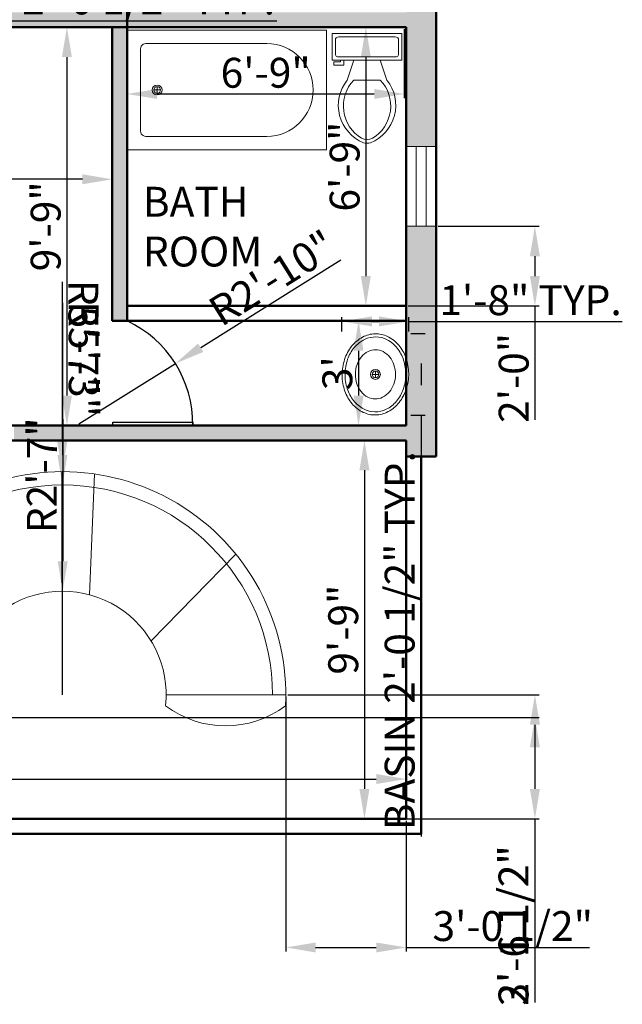
# Model space of a CAD drawing. Units: inches. Extents: x 875413 to 876020, y 447446 to 448210.
# Tile 4 of 8: x 875810 to 875992, y 447498 to 447795. Entities that reach past the tile are written whole.
import ezdxf

# ---------------------------------------------------------------- set-up
doc = ezdxf.new("R2010")
doc.units = ezdxf.units.IN
for name, color, linetype, lineweight in [('A-ANNO-DIMS', 2, 'Continuous', 13), ('A-AREA-IDEN', 7, 'Continuous', 25), ('A-DOOR', 3, 'Continuous', 25), ('A-FLOR-FIXT', 9, 'Continuous', 18), ('A-FURN', 8, 'Continuous', 18), ('A-GLAZ', 4, 'Continuous', 20), ('A-WALL', 7, 'Continuous', 50)]:
    doc.layers.add(name, color=color, linetype=linetype, lineweight=lineweight)
doc.layers.add('A-WALL-PATT', color=18, linetype='Continuous', lineweight=13, true_color=0x000000)
doc.styles.get("Standard").update_dxf_attribs({"font": 'arial.ttf'})
doc.dimstyles.new('ISO-25', dxfattribs={"dimtxt": 9, "dimasz": 9, "dimexe": 1.25, "dimexo": 0.625, "dimtad": 1, "dimdec": 1, "dimrnd": 9, "dimlunit": 3, "dimtxsty": 'Standard', "dimcen": 2.5, "dimadec": 0, "dimazin": 0, "dimtfac": 1, "dimtdec": 1, "dimtmove": 0, "dimatfit": 3, "dimfxl": 1, "dimarcsym": 0})

# ---------------------------------------------------------------- blocks, each defined once
blk = doc.blocks.new('*D19')
at = {"layer": 'A-ANNO-DIMS', "color": 0, "lineweight": -2, "transparency": 16777216}
for p, q in [((875643.2, 447554.64), (875643.2, 447567.26)), ((875652.2, 447566.01), (875917.7, 447566.01)), ((875926.7, 447554.64), (875926.7, 447567.26))]:
    blk.add_line(p, q, dxfattribs=at)
at = {"layer": 'A-ANNO-DIMS', "color": 0, "transparency": 16777216}
for points in [[(875652.2, 447567.51), (875652.2, 447564.51), (875643.2, 447566.01)], [(875917.7, 447567.51), (875917.7, 447564.51), (875926.7, 447566.01)]]:
    blk.add_solid(points, dxfattribs=at)
at = {"layer": 'Defpoints', "color": 0, "transparency": 16777216}
for p in [(875926.7, 447566.01), (875643.2, 447554.02), (875926.7, 447554.02)]:
    blk.add_point(p, dxfattribs=at)
at = {"layer": 'A-ANNO-DIMS', "color": 0, "transparency": 16777216, "insert": (875784.95, 447571.15), "char_height": 9, "attachment_point": 5}
blk.add_mtext("24'", dxfattribs=at)
blk = doc.blocks.new('*D20')
at = {"layer": 'A-ANNO-DIMS', "color": 0, "lineweight": -2, "transparency": 16777216}
for p, q in [((875926.08, 447668.02), (875912.88, 447668.02)), ((875914.13, 447659.02), (875914.13, 447563.02)), ((875926.08, 447554.02), (875912.88, 447554.02))]:
    blk.add_line(p, q, dxfattribs=at)
at = {"layer": 'A-ANNO-DIMS', "color": 0, "transparency": 16777216}
for points in [[(875912.63, 447659.02), (875915.63, 447659.02), (875914.13, 447668.02)], [(875912.63, 447563.02), (875915.63, 447563.02), (875914.13, 447554.02)]]:
    blk.add_solid(points, dxfattribs=at)
at = {"layer": 'Defpoints', "color": 0, "transparency": 16777216}
for p in [(875926.7, 447668.02), (875914.13, 447554.02), (875926.7, 447554.02)]:
    blk.add_point(p, dxfattribs=at)
at = {"layer": 'A-ANNO-DIMS', "color": 0, "transparency": 16777216, "insert": (875908.91, 447611.02), "char_height": 9, "attachment_point": 5, "rotation": 90}
blk.add_mtext('9\'-9"', dxfattribs=at)
blk = doc.blocks.new('*D21')
at = {"layer": 'A-ANNO-DIMS', "color": 0, "lineweight": -2, "transparency": 16777216}
for p, q in [((875926.08, 447792.52), (875913.3, 447792.52)), ((875914.55, 447783.52), (875914.55, 447717.52)), ((875926.08, 447708.52), (875913.3, 447708.52))]:
    blk.add_line(p, q, dxfattribs=at)
at = {"layer": 'A-ANNO-DIMS', "color": 0, "transparency": 16777216}
for points in [[(875913.05, 447783.52), (875916.05, 447783.52), (875914.55, 447792.52)], [(875913.05, 447717.52), (875916.05, 447717.52), (875914.55, 447708.52)]]:
    blk.add_solid(points, dxfattribs=at)
at = {"layer": 'Defpoints', "color": 0, "transparency": 16777216}
for p in [(875926.7, 447792.52), (875914.55, 447708.52), (875926.7, 447708.52)]:
    blk.add_point(p, dxfattribs=at)
at = {"layer": 'A-ANNO-DIMS', "color": 0, "transparency": 16777216, "insert": (875909.33, 447750.52), "char_height": 9, "attachment_point": 5, "rotation": 90}
blk.add_mtext('6\'-9"', dxfattribs=at)
blk = doc.blocks.new('*D22')
at = {"layer": 'A-ANNO-DIMS', "color": 0, "lineweight": -2, "transparency": 16777216}
for p, q in [((875842.7, 447791.89), (875842.7, 447771.14)), ((875926.08, 447791.89), (875926.08, 447771.14)), ((875851.7, 447772.39), (875917.08, 447772.39))]:
    blk.add_line(p, q, dxfattribs=at)
at = {"layer": 'A-ANNO-DIMS', "color": 0, "transparency": 16777216}
for points in [[(875851.7, 447773.89), (875851.7, 447770.89), (875842.7, 447772.39)], [(875917.08, 447773.89), (875917.08, 447770.89), (875926.08, 447772.39)]]:
    blk.add_solid(points, dxfattribs=at)
at = {"layer": 'Defpoints', "color": 0, "transparency": 16777216}
for p in [(875842.7, 447792.52), (875926.08, 447792.52), (875926.08, 447772.39)]:
    blk.add_point(p, dxfattribs=at)
at = {"layer": 'A-ANNO-DIMS', "color": 0, "transparency": 16777216, "insert": (875884.39, 447777.61), "char_height": 9, "attachment_point": 5}
blk.add_mtext('6\'-9"', dxfattribs=at)
blk = doc.blocks.new('*D23')
at = {"layer": 'A-ANNO-DIMS', "color": 0, "lineweight": -2, "transparency": 16777216}
for p, q in [((875926.08, 447704.02), (875911.11, 447704.02)), ((875912.36, 447695.02), (875912.36, 447681.52)), ((875926.08, 447672.52), (875911.11, 447672.52))]:
    blk.add_line(p, q, dxfattribs=at)
at = {"layer": 'A-ANNO-DIMS', "color": 0, "transparency": 16777216}
for points in [[(875910.86, 447695.02), (875913.86, 447695.02), (875912.36, 447704.02)], [(875910.86, 447681.52), (875913.86, 447681.52), (875912.36, 447672.52)]]:
    blk.add_solid(points, dxfattribs=at)
at = {"layer": 'Defpoints', "color": 0, "transparency": 16777216}
for p in [(875926.7, 447704.02), (875912.36, 447672.52), (875926.7, 447672.52)]:
    blk.add_point(p, dxfattribs=at)
at = {"layer": 'A-ANNO-DIMS', "color": 0, "transparency": 16777216, "insert": (875907.14, 447688.27), "char_height": 9, "attachment_point": 5, "rotation": 90}
blk.add_mtext("3'", dxfattribs=at)
blk = doc.blocks.new('*D24')
at = {"layer": 'A-ANNO-DIMS', "color": 0, "lineweight": -2, "transparency": 16777216}
for p, q in [((875689.7, 447791.89), (875689.7, 447745.44)), ((875838.2, 447791.89), (875838.2, 447745.44)), ((875829.2, 447746.69), (875698.7, 447746.69))]:
    blk.add_line(p, q, dxfattribs=at)
at = {"layer": 'A-ANNO-DIMS', "color": 0, "transparency": 16777216}
for points in [[(875698.7, 447748.19), (875698.7, 447745.19), (875689.7, 447746.69)], [(875829.2, 447748.19), (875829.2, 447745.19), (875838.2, 447746.69)]]:
    blk.add_solid(points, dxfattribs=at)
at = {"layer": 'Defpoints', "color": 0, "transparency": 16777216}
for p in [(875689.7, 447792.52), (875838.2, 447792.52), (875689.7, 447746.69)]:
    blk.add_point(p, dxfattribs=at)
at = {"layer": 'A-ANNO-DIMS', "color": 0, "transparency": 16777216, "insert": (875763.95, 447751.91), "char_height": 9, "attachment_point": 5}
blk.add_mtext('12\'-9"', dxfattribs=at)
blk = doc.blocks.new('*D25')
at = {"layer": 'A-ANNO-DIMS', "color": 0, "lineweight": -2, "transparency": 16777216}
for p, q in [((875837.58, 447792.52), (875823.3, 447792.52)), ((875824.55, 447783.52), (875824.55, 447681.52)), ((875837.58, 447672.52), (875823.3, 447672.52))]:
    blk.add_line(p, q, dxfattribs=at)
at = {"layer": 'A-ANNO-DIMS', "color": 0, "transparency": 16777216}
for points in [[(875823.05, 447783.52), (875826.05, 447783.52), (875824.55, 447792.52)], [(875823.05, 447681.52), (875826.05, 447681.52), (875824.55, 447672.52)]]:
    blk.add_solid(points, dxfattribs=at)
at = {"layer": 'Defpoints', "color": 0, "transparency": 16777216}
for p in [(875838.2, 447792.52), (875824.55, 447672.52), (875838.2, 447672.52)]:
    blk.add_point(p, dxfattribs=at)
at = {"layer": 'A-ANNO-DIMS', "color": 0, "transparency": 16777216, "insert": (875819.33, 447732.52), "char_height": 9, "attachment_point": 5, "rotation": 90}
blk.add_mtext('9\'-9"', dxfattribs=at)
blk = doc.blocks.new('Toilet - top')
for p, q in [((9.5, -6), (9.5, -2)), ((-10, -8.5), (-8, -8.5)), ((-10, -9.5), (-10, -8.5)), ((-8, -8.5), (-8, -8)), ((-7, -8), (-7, -9.5)), ((-4, -8), (-6, -14)), ((4, -8), (6, -14)), ((-7, -9.5), (-10, -9.5)), ((4, -14), (-4, -14))]:
    blk.add_line(p, q)
blk.add_lwpolyline([(10.5, -8), (10.5, 0), (-10.5, 0), (-10.5, -8)], close=True)
for points in [[(-9.5, -2), (-9.5, -6)], [(8.5, -1), (-8.5, -1)], [(-8.5, -7), (8.5, -7)]]:
    blk.add_lwpolyline(points)
for centre, radius, start, end in [((-8.62, -1.88), 0.884, 81.8699, 188.1301), ((8.62, -1.88), 0.884, 351.8699, 98.1301), ((-8.62, -6.12), 0.884, 171.8699, 278.1301), ((8.62, -6.12), 0.884, 261.8699, 8.1301), ((3.52, -21.58), 12.17, 141.4691, 247.9714), ((4.2, -21.82), 11.33, 136.3677, 238.9468), ((-3.52, -21.58), 12.17, 292.0284, 38.5307), ((-4.2, -21.82), 11.33, 301.053, 43.6321), ((0, -27.88), 4, 245.7318, 294.2682), ((0, -29), 4, 254.8605, 285.1395)]:
    blk.add_arc(centre, radius, start, end)
blk = doc.blocks.new('Bath Tub - 26 x 60 in.')
for p, q in [((9, -17), (9, -19)), ((8, -18), (10, -18))]:
    blk.add_line(p, q)
blk.add_lwpolyline([(0, -36), (0, 0), (60, 0), (60, -36)], close=True)
for points in [[(6, -4), (42, -4)], [(4, -30), (4, -6)], [(42, -32), (6, -32)]]:
    blk.add_lwpolyline(points)
for radius in [1.5, 1]:
    blk.add_circle((9, -18), radius)
for centre, radius, start, end in [((5.75, -5.75), 1.77, 81.8699, 188.1301), ((42, -18), 14, 270, 90), ((5.75, -30.25), 1.77, 171.8699, 278.1301)]:
    blk.add_arc(centre, radius, start, end)
blk = doc.blocks.new('Sink - Oval top')
for p, q in [((-1, 0), (1, 0)), ((0, 1), (0, -1))]:
    blk.add_line(p, q)
for points in [[(-12.23, 0.39, 0.117634), (-11.46, -3.36, 0.104469), (-8.88, -6.8, 0.090016), (-5.08, -9.07, 0.08192), (-0.32, -10.02, 0.08192), (4.49, -9.38, 0.090016), (8.42, -7.36, 0.104469), (11.22, -4.09, 0.117634), (12.23, -0.39, 0.117634), (11.46, 3.36, 0.104469), (8.88, 6.8, 0.090016), (5.08, 9.07, 0.08192), (0.32, 10.02, 0.08192), (-4.49, 9.38, 0.090016), (-8.42, 7.36, 0.104469), (-11.22, 4.09, 0.117634)], [(-11.29, 0.16, 0.118622), (-10.52, -3.25, 0.104678), (-8.07, -6.36, 0.089562), (-4.54, -8.37, 0.081185), (-0.13, -9.15, 0.081185), (4.3, -8.49, 0.089562), (7.89, -6.58, 0.104678), (10.42, -3.55, 0.118622), (11.29, -0.16, 0.118622), (10.52, 3.25, 0.104678), (8.07, 6.36, 0.089562), (4.54, 8.37, 0.081185), (0.13, 9.15, 0.081185), (-4.3, 8.49, 0.089562), (-7.89, 6.58, 0.104678), (-10.42, 3.55, 0.118622)], [(-7.42, 0.08, 0.118283), (-6.91, -2.17, 0.104607), (-5.29, -4.21, 0.089718), (-2.97, -5.53, 0.081436), (-0.07, -6.04, 0.081436), (2.84, -5.59, 0.089718), (5.2, -4.33, 0.104607), (6.86, -2.32, 0.118283), (7.42, -0.08, 0.118283), (6.91, 2.17, 0.104607), (5.29, 4.21, 0.089718), (2.97, 5.53, 0.081436), (0.07, 6.04, 0.081436), (-2.84, 5.59, 0.089718), (-5.2, 4.33, 0.104607), (-6.86, 2.32, 0.118283)]]:
    blk.add_lwpolyline(points, format="xyb", close=True)
for radius in [1.5, 1]:
    blk.add_circle((0, 0), radius)
blk = doc.blocks.new('WIN-24IN')
for p, q in [((0, 24), (9, 24)), ((3, 0), (3, 24)), ((6, 0), (6, 24)), ((0, 0), (9, 0))]:
    blk.add_line(p, q)
blk = doc.blocks.new('*D47')
at = {"layer": 'A-ANNO-DIMS', "color": 0, "lineweight": -2, "transparency": 16777216}
for p, q in [((875928.12, 447700.2), (875932.43, 447700.2)), ((875931.18, 447691.2), (875931.18, 447684.65)), ((875928.12, 447675.65), (875932.43, 447675.65)), ((875931.18, 447675.65), (875931.18, 447548.74))]:
    blk.add_line(p, q, dxfattribs=at)
at = {"layer": 'A-ANNO-DIMS', "color": 0, "transparency": 16777216}
for points in [[(875929.68, 447691.2), (875932.68, 447691.2), (875931.18, 447700.2)], [(875929.68, 447684.65), (875932.68, 447684.65), (875931.18, 447675.65)]]:
    blk.add_solid(points, dxfattribs=at)
at = {"layer": 'Defpoints', "color": 0, "transparency": 16777216}
for p in [(875927.5, 447700.2), (875927.5, 447675.65), (875931.18, 447675.65)]:
    blk.add_point(p, dxfattribs=at)
at = {"layer": 'A-ANNO-DIMS', "color": 0, "transparency": 16777216, "insert": (875925.9, 447607.69), "char_height": 9, "attachment_point": 5, "rotation": 90}
blk.add_mtext('BASIN 2\'-0 1/2" TYP.', dxfattribs=at)
blk = doc.blocks.new('*D48')
at = {"layer": 'A-ANNO-DIMS', "color": 0, "lineweight": -2, "transparency": 16777216}
for p, q in [((875907.36, 447700.82), (875907.36, 447705.13)), ((875916.36, 447703.88), (875918.5, 447703.88)), ((875927.5, 447700.82), (875927.5, 447705.13)), ((875927.5, 447703.88), (875991.76, 447703.88))]:
    blk.add_line(p, q, dxfattribs=at)
at = {"layer": 'A-ANNO-DIMS', "color": 0, "transparency": 16777216}
for points in [[(875916.36, 447705.38), (875916.36, 447702.38), (875907.36, 447703.88)], [(875918.5, 447705.38), (875918.5, 447702.38), (875927.5, 447703.88)]]:
    blk.add_solid(points, dxfattribs=at)
at = {"layer": 'Defpoints', "color": 0, "transparency": 16777216}
for p in [(875927.5, 447703.88), (875907.36, 447700.2), (875927.5, 447700.2)]:
    blk.add_point(p, dxfattribs=at)
at = {"layer": 'A-ANNO-DIMS', "color": 0, "transparency": 16777216, "insert": (875964.13, 447709.1), "char_height": 9, "attachment_point": 5}
blk.add_mtext('1\'-8" TYP.', dxfattribs=at)
blk = doc.blocks.new('*D58')
at = {"layer": 'A-ANNO-DIMS', "color": 0, "lineweight": -2, "transparency": 16777216}
for p, q in [((875777.09, 447790.98), (875777.09, 447795.66)), ((875786.09, 447794.41), (875792.52, 447794.41)), ((875801.52, 447790.98), (875801.52, 447795.66)), ((875801.52, 447794.41), (875887.76, 447794.41))]:
    blk.add_line(p, q, dxfattribs=at)
at = {"layer": 'A-ANNO-DIMS', "color": 0, "transparency": 16777216}
for points in [[(875786.09, 447795.91), (875786.09, 447792.91), (875777.09, 447794.41)], [(875792.52, 447795.91), (875792.52, 447792.91), (875801.52, 447794.41)]]:
    blk.add_solid(points, dxfattribs=at)
at = {"layer": 'Defpoints', "color": 0, "transparency": 16777216}
for p in [(875801.52, 447794.41), (875777.09, 447790.36), (875801.52, 447790.36)]:
    blk.add_point(p, dxfattribs=at)
at = {"layer": 'A-ANNO-DIMS', "color": 0, "transparency": 16777216, "insert": (875849.14, 447799.69), "char_height": 9, "attachment_point": 5}
blk.add_mtext('2\'-0 1/2" TYP.', dxfattribs=at)
blk = doc.blocks.new('*D76')
at = {"layer": 'A-ANNO-DIMS', "color": 0, "lineweight": -2, "transparency": 16777216}
for p, q in [((875936.33, 447732.52), (875966.7, 447732.52)), ((875965.45, 447723.52), (875965.45, 447717.52)), ((875927.33, 447708.52), (875966.7, 447708.52)), ((875965.45, 447708.52), (875965.45, 447674.19))]:
    blk.add_line(p, q, dxfattribs=at)
at = {"layer": 'A-ANNO-DIMS', "color": 0, "transparency": 16777216}
for points in [[(875963.95, 447723.52), (875966.95, 447723.52), (875965.45, 447732.52)], [(875963.95, 447717.52), (875966.95, 447717.52), (875965.45, 447708.52)]]:
    blk.add_solid(points, dxfattribs=at)
at = {"layer": 'Defpoints', "color": 0, "transparency": 16777216}
for p in [(875935.7, 447732.52), (875926.7, 447708.52), (875965.45, 447708.52)]:
    blk.add_point(p, dxfattribs=at)
at = {"layer": 'A-ANNO-DIMS', "color": 0, "transparency": 16777216, "insert": (875960.23, 447686.85), "char_height": 9, "attachment_point": 5, "rotation": 90}
blk.add_mtext('2\'-0"', dxfattribs=at)
blk = doc.blocks.new('*D83')
at = {"layer": 'A-ANNO-DIMS', "color": 0, "lineweight": -2, "transparency": 16777216}
for p, q in [((875497.15, 447584.59), (875966.7, 447584.59)), ((875965.45, 447575.59), (875965.45, 447563.02)), ((875471.33, 447554.02), (875966.7, 447554.02)), ((875965.45, 447554.02), (875965.45, 447498.72))]:
    blk.add_line(p, q, dxfattribs=at)
at = {"layer": 'A-ANNO-DIMS', "color": 0, "transparency": 16777216}
for points in [[(875963.95, 447575.59), (875966.95, 447575.59), (875965.45, 447584.59)], [(875963.95, 447563.02), (875966.95, 447563.02), (875965.45, 447554.02)]]:
    blk.add_solid(points, dxfattribs=at)
at = {"layer": 'Defpoints', "color": 0, "transparency": 16777216}
for p in [(875496.52, 447584.59), (875470.7, 447554.02), (875965.45, 447554.02)]:
    blk.add_point(p, dxfattribs=at)
at = {"layer": 'A-ANNO-DIMS', "color": 0, "transparency": 16777216, "insert": (875960.17, 447521.87), "char_height": 9, "attachment_point": 5, "rotation": 90}
blk.add_mtext('2\'-6 1/2"', dxfattribs=at)
blk = doc.blocks.new('*D84')
at = {"layer": 'A-ANNO-DIMS', "color": 0, "lineweight": -2, "transparency": 16777216}
for p, q in [((875890.44, 447590.76), (875890.44, 447514.02)), ((875926.7, 447553.39), (875926.7, 447514.02)), ((875899.44, 447515.27), (875917.7, 447515.27)), ((875926.7, 447515.27), (875981.84, 447515.27))]:
    blk.add_line(p, q, dxfattribs=at)
at = {"layer": 'A-ANNO-DIMS', "color": 0, "transparency": 16777216}
for points in [[(875899.44, 447516.77), (875899.44, 447513.77), (875890.44, 447515.27)], [(875917.7, 447516.77), (875917.7, 447513.77), (875926.7, 447515.27)]]:
    blk.add_solid(points, dxfattribs=at)
at = {"layer": 'Defpoints', "color": 0, "transparency": 16777216}
for p in [(875890.44, 447591.38), (875926.7, 447554.02), (875926.7, 447515.27)]:
    blk.add_point(p, dxfattribs=at)
at = {"layer": 'A-ANNO-DIMS', "color": 0, "transparency": 16777216, "insert": (875958.77, 447520.55), "char_height": 9, "attachment_point": 5}
blk.add_mtext('3\'-0 1/2"', dxfattribs=at)
blk = doc.blocks.new('*D85')
at = {"layer": 'A-ANNO-DIMS', "color": 0, "lineweight": -2, "transparency": 16777216}
for p, q in [((875891.07, 447591.38), (875966.7, 447591.38)), ((875965.45, 447582.38), (875965.45, 447563.02)), ((875927.33, 447554.02), (875966.7, 447554.02)), ((875965.45, 447554.02), (875965.45, 447498.88))]:
    blk.add_line(p, q, dxfattribs=at)
at = {"layer": 'A-ANNO-DIMS', "color": 0, "transparency": 16777216}
for points in [[(875963.95, 447582.38), (875966.95, 447582.38), (875965.45, 447591.38)], [(875963.95, 447563.02), (875966.95, 447563.02), (875965.45, 447554.02)]]:
    blk.add_solid(points, dxfattribs=at)
at = {"layer": 'Defpoints', "color": 0, "transparency": 16777216}
for p in [(875890.44, 447591.38), (875926.7, 447554.02), (875965.45, 447554.02)]:
    blk.add_point(p, dxfattribs=at)
at = {"layer": 'A-ANNO-DIMS', "color": 0, "transparency": 16777216, "insert": (875960.17, 447521.95), "char_height": 9, "attachment_point": 5, "rotation": 90}
blk.add_mtext('3\'-1 1/2"', dxfattribs=at)
blk = doc.blocks.new('*D88')
at = {"layer": 'A-ANNO-DIMS', "color": 0, "lineweight": -2, "transparency": 16777216}
for p, q in [((875823.11, 447715.84), (875823.15, 447667.61)), ((875823.22, 447591.38), (875823.16, 447658.61))]:
    blk.add_line(p, q, dxfattribs=at)
at = {"layer": 'A-ANNO-DIMS', "color": 0, "transparency": 16777216}
blk.add_solid([(875824.65, 447667.61), (875821.65, 447667.61), (875823.16, 447658.61)], dxfattribs=at)
at = {"layer": 'Defpoints', "color": 0, "transparency": 16777216}
for p in [(875823.16, 447658.61), (875823.22, 447591.38)]:
    blk.add_point(p, dxfattribs=at)
at = {"layer": 'A-ANNO-DIMS', "color": 0, "transparency": 16777216, "insert": (875828.33, 447698.95), "char_height": 9, "attachment_point": 5, "rotation": 270.0471}
blk.add_mtext('R5\'-7"', dxfattribs=at)
blk = doc.blocks.new('*D89')
at = {"layer": 'A-ANNO-DIMS', "color": 0, "lineweight": -2, "transparency": 16777216}
for p, q in [((875823.21, 447709.44), (875823.21, 447663.61)), ((875823.22, 447591.38), (875823.21, 447654.61))]:
    blk.add_line(p, q, dxfattribs=at)
at = {"layer": 'A-ANNO-DIMS', "color": 0, "transparency": 16777216}
blk.add_solid([(875824.71, 447663.61), (875821.71, 447663.61), (875823.21, 447654.61)], dxfattribs=at)
at = {"layer": 'Defpoints', "color": 0, "transparency": 16777216}
for p in [(875823.21, 447654.61), (875823.22, 447591.38)]:
    blk.add_point(p, dxfattribs=at)
at = {"layer": 'A-ANNO-DIMS', "color": 0, "transparency": 16777216, "insert": (875828.44, 447692.54), "char_height": 9, "attachment_point": 5, "rotation": 270.0002}
blk.add_mtext('R5\'-3"', dxfattribs=at)
blk = doc.blocks.new('*D90')
at = {"layer": 'A-ANNO-DIMS', "color": 0, "lineweight": -2, "transparency": 16777216}
for p, q in [((875823.35, 447674.39), (875823.28, 447631.61)), ((875823.22, 447591.38), (875823.27, 447622.61))]:
    blk.add_line(p, q, dxfattribs=at)
at = {"layer": 'A-ANNO-DIMS', "color": 0, "transparency": 16777216}
blk.add_solid([(875821.78, 447631.61), (875824.78, 447631.6), (875823.27, 447622.61)], dxfattribs=at)
at = {"layer": 'Defpoints', "color": 0, "transparency": 16777216}
for p in [(875823.27, 447622.61), (875823.22, 447591.38)]:
    blk.add_point(p, dxfattribs=at)
at = {"layer": 'A-ANNO-DIMS', "color": 0, "transparency": 16777216, "insert": (875818.18, 447657.51), "char_height": 9, "attachment_point": 5, "rotation": 89.9069}
blk.add_mtext('R2\'-7"', dxfattribs=at)
blk = doc.blocks.new('*D96')
at = {"layer": 'A-ANNO-DIMS', "color": 0, "lineweight": -2, "transparency": 16777216}
for p, q in [((875907.03, 447722.36), (875864.84, 447695.95)), ((875828.19, 447673.02), (875857.21, 447691.18))]:
    blk.add_line(p, q, dxfattribs=at)
at = {"layer": 'A-ANNO-DIMS', "color": 0, "transparency": 16777216}
blk.add_solid([(875864.04, 447697.22), (875865.63, 447694.68), (875857.21, 447691.18)], dxfattribs=at)
at = {"layer": 'Defpoints', "color": 0, "transparency": 16777216}
for p in [(875857.21, 447691.18), (875828.19, 447673.02)]:
    blk.add_point(p, dxfattribs=at)
at = {"layer": 'A-ANNO-DIMS', "color": 0, "transparency": 16777216, "insert": (875886.98, 447715.97), "char_height": 9, "attachment_point": 5, "rotation": 32.0401}
blk.add_mtext('R2\'-10"', dxfattribs=at)

msp = doc.modelspace()

# ---------------------------------------------------------------- hatches: boundary and pattern name
at = {"layer": 'A-WALL-PATT'}
h = msp.add_hatch(color=256, dxfattribs=at)
h.dxf.hatch_style = 1
h.paths.add_polyline_path([(875470.7, 447985.13), (875461.7, 447985.13), (875461.7, 447865.29), (875470.7, 447865.29), (875470.7, 447881.02), (875566.7, 447881.02), (875566.7, 447797.02), (875571.2, 447797.02), (875571.2, 447885.52), (875571.2, 447921.52), (875603.29, 447921.52), (875603.29, 447926.02), (875501.27, 447926.02), (875501.27, 447921.52), (875566.7, 447921.52), (875566.7, 447885.52), (875470.7, 447885.52), (875470.7, 447921.52), (875470.7, 447926.02)])
h.paths.add_polyline_path([(875470.7, 448070.02), (875518.96, 448070.02), (875518.96, 448079.02), (875461.7, 448079.02), (875461.7, 448045.13), (875470.7, 448045.13)])
h.paths.add_polyline_path([(875819.9, 448079.02), (875578.96, 448079.02), (875578.96, 448070.02), (875638.7, 448070.02), (875638.7, 447921.52), (875643.2, 447921.52), (875643.2, 448070.02), (875763.2, 448070.02), (875763.2, 447921.52), (875767.7, 447921.52), (875767.7, 448070.02), (875819.9, 448070.02)])
h.paths.add_polyline_path([(875935.7, 447978.92), (875926.7, 447978.92), (875926.7, 447926.02), (875926.7, 447921.52), (875926.7, 447885.52), (875842.7, 447885.52), (875842.7, 447921.52), (875899.7, 447921.52), (875899.7, 447926.02), (875805.34, 447926.02), (875805.34, 447921.52), (875838.2, 447921.52), (875838.2, 447885.52), (875838.2, 447797.02), (875689.7, 447797.02), (875689.7, 447792.52), (875842.7, 447792.52), (875842.7, 447881.02), (875926.7, 447881.02), (875926.7, 447857.16), (875935.7, 447857.16)])
h.paths.add_polyline_path([(875935.7, 448079.02), (875879.9, 448079.02), (875879.9, 448070.02), (875926.7, 448070.02), (875926.7, 448038.92), (875935.7, 448038.92)])
h.paths.add_polyline_path([(875935.7, 447833.16), (875926.7, 447833.16), (875926.7, 447797.02), (875842.7, 447797.02), (875842.7, 447792.52), (875926.7, 447792.52), (875926.7, 447756.52), (875935.7, 447756.52)])
h.paths.add_polyline_path([(875935.7, 447732.52), (875926.7, 447732.52), (875926.7, 447692.75, -0.007222), (875926.81, 447692.41, -0.08192), (875927.45, 447687.6, -0.071798), (875926.7, 447683.4), (875926.7, 447672.52), (875808.63, 447672.52), (875808.63, 447668.02), (875926.7, 447668.02), (875926.7, 447663.19), (875935.7, 447663.19)])
h.paths.add_polyline_path([(875842.7, 447792.52), (875838.2, 447792.52), (875838.2, 447704.02), (875842.7, 447704.02)])
h.paths.add_polyline_path([(875470.7, 447792.52), (875619.2, 447792.52), (875619.2, 447797.02), (875470.7, 447797.02), (875470.7, 447841.29), (875461.7, 447841.29), (875461.7, 447764.71), (875470.7, 447764.71)])
h.paths.add_polyline_path([(875619.2, 447760.51), (875616.95, 447760.51, -0.018388), (875614.7, 447760.37), (875614.7, 447672.52), (875470.7, 447672.52), (875470.7, 447704.71), (875461.7, 447704.71), (875461.7, 447640.7), (875470.7, 447640.7), (875470.7, 447668.02), (875619.2, 447668.02)])
h.paths.add_polyline_path([(875511.12, 447554.02), (875470.7, 447554.02), (875470.7, 447580.7), (875461.7, 447580.7), (875461.7, 447545.02), (875511.12, 447545.02)])
h.paths.add_polyline_path([(875656.47, 447554.02), (875620.05, 447554.02, -0.057036), (875616.67, 447553.74, -0.040891), (875614.26, 447554.02), (875571.12, 447554.02), (875571.12, 447545.02), (875656.47, 447545.02)])
h.paths.add_polyline_path([(875643.2, 447613.27), (875685.21, 447613.27), (875685.21, 447617.77), (875685.21, 447623.8), (875680.71, 447623.8), (875680.71, 447617.77), (875618.23, 447617.77), (875618.23, 447623.8), (875613.73, 447623.8), (875613.73, 447617.77), (875613.73, 447613.27), (875638.7, 447613.27), (875638.7, 447554.02), (875643.2, 447554.02)])
h.paths.add_polyline_path([(875694.2, 447760.28), (875689.7, 447760.28), (875689.7, 447668.02), (875748.63, 447668.02), (875748.63, 447672.52), (875694.2, 447672.52)])

# ---------------------------------------------------------------- linework, layer by layer
at = {"layer": 'A-DOOR'}
for p, q in [((875838.42, 447672.52), (875838.42, 447673.52)), ((875838.42, 447673.52), (875862.42, 447673.52)), ((875862.42, 447673.52), (875862.42, 447672.52))]:
    msp.add_line(p, q, dxfattribs=at)
msp.add_arc((875828.19, 447673.02), 34.23, 359.163, 64.9166, dxfattribs=at)
at = {"layer": 'A-FURN'}
for p, q in [((875831.32, 447621.54), (875832.84, 447657.91)), ((875849.89, 447607.62), (875875.42, 447633.74)), ((875890.44, 447591.38), (875854.44, 447591.38))]:
    msp.add_line(p, q, dxfattribs=at)
for centre, radius, start, end in [((875823.22, 447591.38), 67.23, 357.2076, 182.8871), ((875823.22, 447591.38), 63.23, 0, 180), ((875823.22, 447591.38), 31.23, 354.002, 185.813), ((875872.32, 447611.83), 29.81, 232.7197, 307.2415)]:
    msp.add_arc(centre, radius, start, end, dxfattribs=at)
at = {"layer": 'A-WALL'}
for p, q in [((875935.7, 447663.19), (875935.7, 448079.02)), ((875842.7, 447704.02), (875842.7, 447881.02)), ((875926.7, 447792.52), (875689.7, 447792.52)), ((875838.2, 447704.02), (875838.2, 447792.52)), ((875926.7, 447672.52), (875926.7, 447792.52)), ((875926.7, 447708.52), (875842.7, 447708.52)), ((875926.7, 447704.02), (875838.2, 447704.02)), ((875926.7, 447672.52), (875694.2, 447672.52)), ((875926.7, 447668.02), (875689.7, 447668.02)), ((875926.7, 447663.19), (875926.7, 447668.02)), ((875926.7, 447663.19), (875935.7, 447663.19)), ((875926.7, 447554.02), (875926.7, 447663.19)), ((875931.2, 447549.52), (875931.2, 447663.19)), ((875656.47, 447554.02), (875926.7, 447554.02)), ((875656.47, 447549.52), (875931.2, 447549.52))]:
    msp.add_line(p, q, dxfattribs=at)

# ---------------------------------------------------------------- block references
at = {"layer": 'A-FLOR-FIXT'}
for name, p in [('Bath Tub - 26 x 60 in.', (875842.7, 447791.59)), ('Toilet - top', (875914.91, 447790.56))]:
    msp.add_blockref(name, p, dxfattribs=at)
at = {"layer": 'A-FLOR-FIXT', "rotation": 270}
msp.add_blockref('Sink - Oval top', (875917.43, 447687.92), dxfattribs=at)
at = {"layer": 'A-GLAZ'}
msp.add_blockref('WIN-24IN', (875926.7, 447732.52), dxfattribs=at)

# ---------------------------------------------------------------- texts
at = {"layer": 'A-AREA-IDEN', "insert": (875847.42, 447744.42), "char_height": 9, "attachment_point": 1}
msp.add_mtext_dynamic_manual_height_columns('BATH\\PROOM', width=100.7812, gutter_width=12.5, heights=[0], dxfattribs=at)

# ---------------------------------------------------------------- dimensions: what is measured, and where the dimension line sits
at = {"layer": 'A-ANNO-DIMS'}
for base, p1, p2, picture, middle in [((875801.52, 447794.41), (875777.09, 447790.36), (875801.52, 447790.36), '*D58', (875849.14, 447799.69)), ((875927.5, 447703.88), (875907.36, 447700.2), (875927.5, 447700.2), '*D48', (875964.13, 447709.1))]:
    dim = msp.add_linear_dim(base=base, p1=p1, p2=p2, text='<> TYP.', dimstyle='ISO-25', override={"dimdec": 1, "dimlfac": 1, "dimrnd": 0, "dimzin": 1, "dimdsep": 46, "dimlunit": 4, "dimfrac": 2}, dxfattribs=at)
    dim.commit()
    dim.dimension.update_dxf_attribs({"geometry": picture, "text_midpoint": middle})
for base, p1, p2, override, picture, middle in [((875689.7, 447746.69), (875838.2, 447792.52), (875689.7, 447792.52), {"dimclrd": 0, "dimclre": 0, "dimclrt": 0}, '*D24', (875763.95, 447751.91)), ((875926.08, 447772.39), (875842.7, 447792.52), (875926.08, 447792.52), {"dimclrd": 0, "dimclre": 0, "dimclrt": 0}, '*D22', (875884.39, 447777.61)), ((875926.7, 447515.27), (875890.44, 447591.38), (875926.7, 447554.02), {"dimdec": 1, "dimlfac": 1, "dimrnd": 0, "dimzin": 1, "dimdsep": 46, "dimlunit": 4, "dimfrac": 2}, '*D84', (875958.77, 447520.55)), ((875926.7, 447566.01), (875643.2, 447554.02), (875926.7, 447554.02), {"dimclrd": 0, "dimclre": 0, "dimclrt": 0}, '*D19', (875784.95, 447571.15))]:
    dim = msp.add_linear_dim(base=base, p1=p1, p2=p2, dimstyle='ISO-25', override=override, dxfattribs=at)
    dim.commit()
    dim.dimension.update_dxf_attribs({"geometry": picture, "text_midpoint": middle})
for base, p1, p2, override, picture, middle in [((875824.55, 447672.52), (875838.2, 447792.52), (875838.2, 447672.52), {"dimclrd": 0, "dimclre": 0, "dimclrt": 0}, '*D25', (875819.33, 447732.52)), ((875914.55, 447708.52), (875926.7, 447792.52), (875926.7, 447708.52), {"dimclrd": 0, "dimclre": 0, "dimclrt": 0}, '*D21', (875909.33, 447750.52)), ((875965.45, 447708.52), (875935.7, 447732.52), (875926.7, 447708.52), {"dimdec": 1, "dimlfac": 1, "dimrnd": 0, "dimzin": 1, "dimdsep": 46, "dimlunit": 4, "dimfrac": 2}, '*D76', (875960.23, 447686.85)), ((875912.36, 447672.52), (875926.7, 447704.02), (875926.7, 447672.52), {"dimclrd": 0, "dimclre": 0, "dimclrt": 0}, '*D23', (875907.14, 447688.27)), ((875914.13, 447554.02), (875926.7, 447668.02), (875926.7, 447554.02), {"dimclrd": 0, "dimclre": 0, "dimclrt": 0}, '*D20', (875908.91, 447611.02)), ((875965.45, 447554.02), (875890.44, 447591.38), (875926.7, 447554.02), {"dimdec": 1, "dimlfac": 1, "dimrnd": 0, "dimzin": 1, "dimdsep": 46, "dimlunit": 4, "dimfrac": 2}, '*D85', (875960.17, 447521.95)), ((875965.45, 447554.02), (875496.52, 447584.59), (875470.7, 447554.02), {"dimdec": 1, "dimlfac": 1, "dimrnd": 0, "dimzin": 1, "dimdsep": 46, "dimlunit": 4, "dimfrac": 2}, '*D83', (875960.17, 447521.87))]:
    dim = msp.add_linear_dim(base=base, p1=p1, p2=p2, angle=90, dimstyle='ISO-25', override=override, dxfattribs=at)
    dim.commit()
    dim.dimension.update_dxf_attribs({"geometry": picture, "text_midpoint": middle})
for center, mpoint, picture, middle in [((875828.19, 447673.02), (875857.21, 447691.18), '*D96', (875886.98, 447715.97)), ((875823.22, 447591.38), (875823.27, 447622.61), '*D90', (875818.18, 447657.51))]:
    dim = msp.add_radius_dim(center=center, mpoint=mpoint, dimstyle='ISO-25', override={"dimdec": 1, "dimlfac": 1, "dimrnd": 0, "dimzin": 1, "dimdsep": 46, "dimlunit": 4, "dimfrac": 2}, dxfattribs=at)
    dim.commit()
    dim.dimension.update_dxf_attribs({"geometry": picture, "text_midpoint": middle})
for mpoint, picture, middle in [((875823.16, 447658.61), '*D88', (875823.13, 447698.94)), ((875823.22, 447654.61), '*D89', (875823.21, 447692.54))]:
    dim = msp.add_radius_dim(center=(875823.22, 447591.38), mpoint=mpoint, dimstyle='ISO-25', override={"dimdec": 1, "dimlfac": 1, "dimrnd": 0, "dimzin": 1, "dimdsep": 46, "dimlunit": 4, "dimfrac": 2}, dxfattribs=at)
    dim.commit()
    dim.dimension.update_dxf_attribs({"geometry": picture, "text_midpoint": middle, "dimtype": 164})
dim = msp.add_linear_dim(base=(875931.1814, 447675.6455), p1=(875927.4988, 447700.1964), p2=(875927.4988, 447675.6455), angle=270, text='BASIN <> TYP.', dimstyle='ISO-25', override={"dimdec": 1, "dimlfac": 1, "dimrnd": 0, "dimzin": 1, "dimdsep": 46, "dimlunit": 4, "dimfrac": 2}, dxfattribs=at)
dim.commit()
dim.dimension.update_dxf_attribs({"geometry": '*D47', "text_midpoint": (875925.9029, 447607.6924)})

doc.saveas('drawing.dxf')
